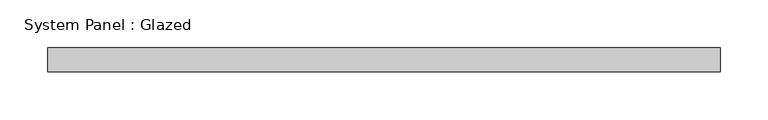
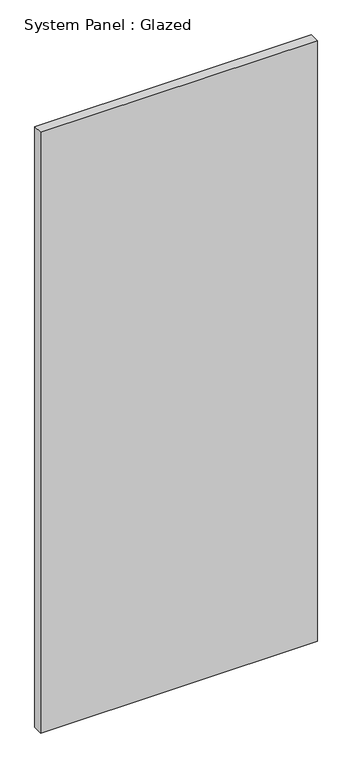
"""IFC4 building model written with IfcOpenShell, lengths in millimetres: plate geometry, System Panel : Glazed."""

from ifc_helpers import new_model, si_unit, origin, origin_with_axes, place, context, project, spatial, polyline, outline, extrude, source, transform, mapped, element, save


def system_panel_glazed_73ac8250(model_context):
    return source(origin(), model_context, "Body", "SweptSolid", [
        extrude(outline(polyline([(352.425, 19.05), (-352.425, 19.05), (-352.425, 44.45), (352.425, 44.45), (352.425, 19.05)])), origin_with_axes(), (0.0, 0.0, 1.0), 1617.0799136),
    ])


if __name__ == "__main__":
    model = new_model("IFC4")
    model_context = context("Model", 3, world=origin())
    ifc_project = project(units=[si_unit("LENGTHUNIT", "METRE", prefix="MILLI")], contexts=[model_context])
    site = spatial("IfcSite", under=ifc_project)
    building = spatial("IfcBuilding", under=site)
    placement = place(None, origin())
    system_panel_glazed_shape = system_panel_glazed_73ac8250(model_context)
    element("IfcPlate", 1, ObjectType="System Panel : Glazed", at=placement, inside=building, context=model_context, shape_type="MappedRepresentation", body=[
        mapped(system_panel_glazed_shape, transform((0.0, 0.0, 0.0), x_axis=(1.0, 0.0, 0.0), y_axis=(0.0, 1.0, 0.0), z_axis=(0.0, 0.0, 1.0))),
    ])
    save(model, "model.ifc")

# Revit data of these elements
# Type "System Panel : Glazed"
#   Construction Type Id = "GSP4R"
#   Analytic Construction = "1/8 in Pilkington single glazing"
#   Visual Light Transmittance = 0.9
#   Solar Heat Gain Coefficient = 0.86
#   Heat Transfer Coefficient (U) = 1.18115 BTU/(h·ft²·°F)
#   Define Thermal Properties by = 1
# Element 1 (IfcPlate, "System Panel : Glazed")
#   Materials on its faces: "Glass"
# Materials
#   "Glass": class "Glass", colour RGB 0 128 192, transparency 0.75, Description = "Soda Lime Glass", Cost = 0
